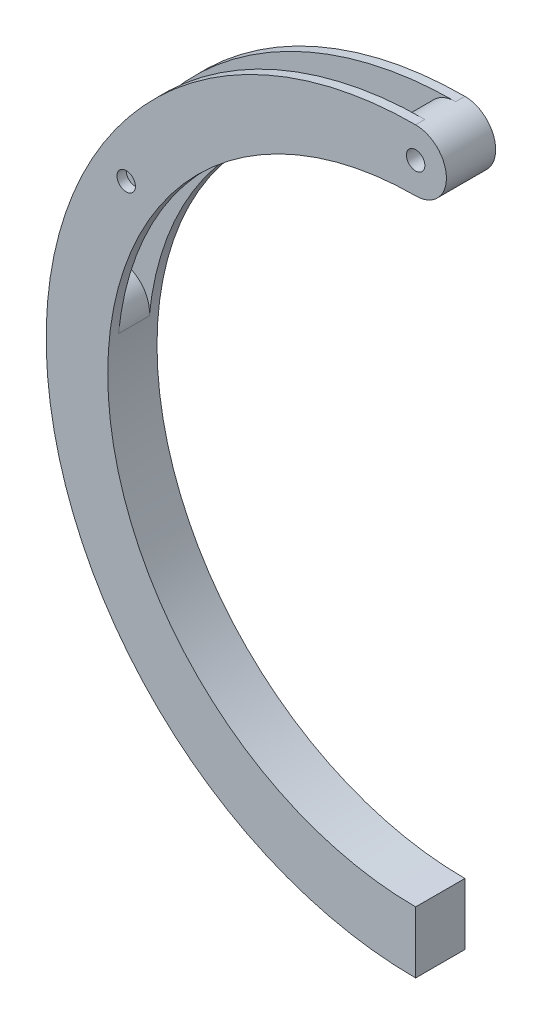
ISO-10303-21;
HEADER;
FILE_DESCRIPTION(('STEP AP214'),'2;1');
FILE_NAME('part.step','',(''),(''),'','','');
FILE_SCHEMA(('AUTOMOTIVE_DESIGN { 1 0 10303 214 1 1 1 1 }'));
ENDSEC;
DATA;
#1=APPLICATION_CONTEXT('core data for automotive mechanical design processes');
#2=APPLICATION_PROTOCOL_DEFINITION('international standard','automotive_design',2000,#1);
#3=PRODUCT_CONTEXT('',#1,'mechanical');
#4=PRODUCT('Part','Part','',(#3));
#5=PRODUCT_RELATED_PRODUCT_CATEGORY('part','',(#4));
#6=PRODUCT_DEFINITION_FORMATION('','',#4);
#7=PRODUCT_DEFINITION_CONTEXT('part definition',#1,'design');
#8=PRODUCT_DEFINITION('design','',#6,#7);
#9=PRODUCT_DEFINITION_SHAPE('','',#8);
#10=(LENGTH_UNIT() NAMED_UNIT(*) SI_UNIT(.MILLI.,.METRE.));
#11=(NAMED_UNIT(*) PLANE_ANGLE_UNIT() SI_UNIT($,.RADIAN.));
#12=(NAMED_UNIT(*) SI_UNIT($,.STERADIAN.) SOLID_ANGLE_UNIT());
#13=UNCERTAINTY_MEASURE_WITH_UNIT(LENGTH_MEASURE(1.E-05),#10,'distance_accuracy_value','');
#14=(GEOMETRIC_REPRESENTATION_CONTEXT(3) GLOBAL_UNCERTAINTY_ASSIGNED_CONTEXT((#13)) GLOBAL_UNIT_ASSIGNED_CONTEXT((#10,
#11,#12)) REPRESENTATION_CONTEXT('',''));
#15=CARTESIAN_POINT('',(0.,0.,0.));
#16=DIRECTION('',(0.,0.,1.));
#17=DIRECTION('',(1.,0.,0.));
#18=AXIS2_PLACEMENT_3D('',#15,#16,#17);
#19=CARTESIAN_POINT('',(0.,0.,4.));
#20=DIRECTION('',(0.,0.,1.));
#21=DIRECTION('',(1.,0.,0.));
#22=AXIS2_PLACEMENT_3D('',#19,#20,#21);
#23=PLANE('',#22);
#24=CARTESIAN_POINT('',(-47.,28.5657137141714,4.));
#25=DIRECTION('',(0.,0.,1.));
#26=DIRECTION('',(1.,0.,0.));
#27=AXIS2_PLACEMENT_3D('',#24,#25,#26);
#28=CIRCLE('',#27,1.5);
#29=CARTESIAN_POINT('',(-45.5,28.5657137141714,4.));
#30=VERTEX_POINT('',#29);
#31=EDGE_CURVE('E125',#30,#30,#28,.T.);
#32=ORIENTED_EDGE('',*,*,#31,.F.);
#33=EDGE_LOOP('',(#32));
#34=FACE_BOUND('',#33,.T.);
#35=CARTESIAN_POINT('',(0.,0.,4.));
#36=DIRECTION('',(0.,0.,1.));
#37=DIRECTION('',(1.,0.,0.));
#38=AXIS2_PLACEMENT_3D('',#35,#36,#37);
#39=CIRCLE('',#38,60.);
#40=CARTESIAN_POINT('',(0.,60.,4.));
#41=VERTEX_POINT('',#40);
#42=CARTESIAN_POINT('',(0.,-60.,4.));
#43=VERTEX_POINT('',#42);
#44=EDGE_CURVE('E123',#41,#43,#39,.T.);
#45=ORIENTED_EDGE('',*,*,#44,.T.);
#46=DIRECTION('',(0.,1.,0.));
#47=VECTOR('',#46,1.);
#48=CARTESIAN_POINT('',(0.,-50.,4.));
#49=LINE('',#48,#47);
#50=CARTESIAN_POINT('',(0.,-50.,4.));
#51=VERTEX_POINT('',#50);
#52=EDGE_CURVE('E186',#43,#51,#49,.T.);
#53=ORIENTED_EDGE('',*,*,#52,.T.);
#54=CARTESIAN_POINT('',(0.,0.,4.));
#55=DIRECTION('',(0.,0.,-1.));
#56=DIRECTION('',(1.,0.,0.));
#57=AXIS2_PLACEMENT_3D('',#54,#55,#56);
#58=CIRCLE('',#57,50.);
#59=CARTESIAN_POINT('',(0.,50.,4.));
#60=VERTEX_POINT('',#59);
#61=EDGE_CURVE('E150',#51,#60,#58,.T.);
#62=ORIENTED_EDGE('',*,*,#61,.T.);
#63=CARTESIAN_POINT('',(0.,55.,4.));
#64=DIRECTION('',(0.,0.,1.));
#65=DIRECTION('',(-1.,0.,0.));
#66=AXIS2_PLACEMENT_3D('',#63,#64,#65);
#67=CIRCLE('',#66,5.);
#68=EDGE_CURVE('E133',#60,#41,#67,.T.);
#69=ORIENTED_EDGE('',*,*,#68,.T.);
#70=EDGE_LOOP('',(#45,#53,#62,#69));
#71=FACE_BOUND('',#70,.T.);
#72=CARTESIAN_POINT('',(0.,55.,4.));
#73=DIRECTION('',(0.,0.,1.));
#74=DIRECTION('',(1.,0.,0.));
#75=AXIS2_PLACEMENT_3D('',#72,#73,#74);
#76=CIRCLE('',#75,1.5);
#77=CARTESIAN_POINT('',(1.5,55.,4.));
#78=VERTEX_POINT('',#77);
#79=EDGE_CURVE('E176',#78,#78,#76,.T.);
#80=ORIENTED_EDGE('',*,*,#79,.F.);
#81=EDGE_LOOP('',(#80));
#82=FACE_BOUND('',#81,.T.);
#83=ADVANCED_FACE('F39',(#34,#71,#82),#23,.T.);
#84=CARTESIAN_POINT('',(0.,0.,2.5));
#85=DIRECTION('',(0.,0.,1.));
#86=DIRECTION('',(1.,0.,0.));
#87=AXIS2_PLACEMENT_3D('',#84,#85,#86);
#88=PLANE('',#87);
#89=CARTESIAN_POINT('',(-54.7247707207909,5.49540440339574,2.5));
#90=DIRECTION('',(0.,0.,1.));
#91=DIRECTION('',(1.,0.,0.));
#92=AXIS2_PLACEMENT_3D('',#89,#90,#91);
#93=CIRCLE('',#92,4.99999999999999);
#94=CARTESIAN_POINT('',(-49.7497915643554,4.99582218490522,2.5));
#95=VERTEX_POINT('',#94);
#96=CARTESIAN_POINT('',(-59.6997498772265,5.99498662188626,2.5));
#97=VERTEX_POINT('',#96);
#98=EDGE_CURVE('E53',#95,#97,#93,.T.);
#99=ORIENTED_EDGE('',*,*,#98,.T.);
#100=CARTESIAN_POINT('',(0.,0.,2.5));
#101=DIRECTION('',(0.,0.,1.));
#102=DIRECTION('',(1.,0.,0.));
#103=AXIS2_PLACEMENT_3D('',#100,#101,#102);
#104=CIRCLE('',#103,60.);
#105=CARTESIAN_POINT('',(0.,60.,2.5));
#106=VERTEX_POINT('',#105);
#107=EDGE_CURVE('E113',#106,#97,#104,.T.);
#108=ORIENTED_EDGE('',*,*,#107,.F.);
#109=CARTESIAN_POINT('',(0.,55.,2.5));
#110=DIRECTION('',(0.,0.,1.));
#111=DIRECTION('',(1.,0.,0.));
#112=AXIS2_PLACEMENT_3D('',#109,#110,#111);
#113=CIRCLE('',#112,5.);
#114=CARTESIAN_POINT('',(0.,50.,2.5));
#115=VERTEX_POINT('',#114);
#116=EDGE_CURVE('E179',#106,#115,#113,.T.);
#117=ORIENTED_EDGE('',*,*,#116,.T.);
#118=CARTESIAN_POINT('',(0.,0.,2.5));
#119=DIRECTION('',(0.,0.,-1.));
#120=DIRECTION('',(1.,0.,0.));
#121=AXIS2_PLACEMENT_3D('',#118,#119,#120);
#122=CIRCLE('',#121,50.);
#123=EDGE_CURVE('E118',#95,#115,#122,.T.);
#124=ORIENTED_EDGE('',*,*,#123,.F.);
#125=EDGE_LOOP('',(#99,#108,#117,#124));
#126=FACE_BOUND('',#125,.T.);
#127=CARTESIAN_POINT('',(-47.,28.5657137141714,2.5));
#128=DIRECTION('',(0.,0.,1.));
#129=DIRECTION('',(1.,0.,0.));
#130=AXIS2_PLACEMENT_3D('',#127,#128,#129);
#131=CIRCLE('',#130,1.5);
#132=CARTESIAN_POINT('',(-45.5,28.5657137141714,2.5));
#133=VERTEX_POINT('',#132);
#134=EDGE_CURVE('E126',#133,#133,#131,.T.);
#135=ORIENTED_EDGE('',*,*,#134,.T.);
#136=EDGE_LOOP('',(#135));
#137=FACE_BOUND('',#136,.T.);
#138=ADVANCED_FACE('F115',(#126,#137),#88,.F.);
#139=CARTESIAN_POINT('',(0.,0.,4.));
#140=DIRECTION('',(0.,0.,-1.));
#141=DIRECTION('',(-1.,0.,0.));
#142=AXIS2_PLACEMENT_3D('',#139,#140,#141);
#143=CYLINDRICAL_SURFACE('',#142,60.);
#144=ORIENTED_EDGE('',*,*,#107,.T.);
#145=DIRECTION('',(0.,0.,-1.));
#146=VECTOR('',#145,1.);
#147=CARTESIAN_POINT('',(-59.6997498772265,5.99498662188626,95.0721450653398));
#148=LINE('',#147,#146);
#149=CARTESIAN_POINT('',(-59.6997498772265,5.99498662188626,-2.5));
#150=VERTEX_POINT('',#149);
#151=EDGE_CURVE('E105',#97,#150,#148,.T.);
#152=ORIENTED_EDGE('',*,*,#151,.T.);
#153=CARTESIAN_POINT('',(0.,0.,-2.5));
#154=DIRECTION('',(0.,0.,1.));
#155=DIRECTION('',(1.,0.,0.));
#156=AXIS2_PLACEMENT_3D('',#153,#154,#155);
#157=CIRCLE('',#156,60.);
#158=CARTESIAN_POINT('',(0.,60.,-2.5));
#159=VERTEX_POINT('',#158);
#160=EDGE_CURVE('E65',#159,#150,#157,.T.);
#161=ORIENTED_EDGE('',*,*,#160,.F.);
#162=DIRECTION('',(0.,0.,1.));
#163=VECTOR('',#162,1.);
#164=CARTESIAN_POINT('',(0.,60.,-4.));
#165=LINE('',#164,#163);
#166=CARTESIAN_POINT('',(0.,60.,-4.));
#167=VERTEX_POINT('',#166);
#168=EDGE_CURVE('E175',#167,#159,#165,.T.);
#169=ORIENTED_EDGE('',*,*,#168,.F.);
#170=CARTESIAN_POINT('',(0.,0.,-4.));
#171=DIRECTION('',(0.,0.,1.));
#172=DIRECTION('',(1.,0.,0.));
#173=AXIS2_PLACEMENT_3D('',#170,#171,#172);
#174=CIRCLE('',#173,60.);
#175=CARTESIAN_POINT('',(0.,-60.,-4.));
#176=VERTEX_POINT('',#175);
#177=EDGE_CURVE('E161',#167,#176,#174,.T.);
#178=ORIENTED_EDGE('',*,*,#177,.T.);
#179=DIRECTION('',(0.,0.,-1.));
#180=VECTOR('',#179,1.);
#181=CARTESIAN_POINT('',(0.,-60.,4.));
#182=LINE('',#181,#180);
#183=EDGE_CURVE('E11',#43,#176,#182,.T.);
#184=ORIENTED_EDGE('',*,*,#183,.F.);
#185=ORIENTED_EDGE('',*,*,#44,.F.);
#186=DIRECTION('',(0.,0.,-1.));
#187=VECTOR('',#186,1.);
#188=CARTESIAN_POINT('',(0.,60.,4.));
#189=LINE('',#188,#187);
#190=EDGE_CURVE('E124',#41,#106,#189,.T.);
#191=ORIENTED_EDGE('',*,*,#190,.T.);
#192=EDGE_LOOP('',(#144,#152,#161,#169,#178,#184,#185,#191));
#193=FACE_BOUND('',#192,.T.);
#194=ADVANCED_FACE('F41',(#193),#143,.T.);
#195=CARTESIAN_POINT('',(0.,-50.,4.));
#196=DIRECTION('',(-1.,0.,0.));
#197=DIRECTION('',(0.,0.,1.));
#198=AXIS2_PLACEMENT_3D('',#195,#196,#197);
#199=PLANE('',#198);
#200=ORIENTED_EDGE('',*,*,#183,.T.);
#201=DIRECTION('',(0.,1.,0.));
#202=VECTOR('',#201,1.);
#203=CARTESIAN_POINT('',(0.,-50.,-4.));
#204=LINE('',#203,#202);
#205=CARTESIAN_POINT('',(0.,-50.,-4.));
#206=VERTEX_POINT('',#205);
#207=EDGE_CURVE('E152',#176,#206,#204,.T.);
#208=ORIENTED_EDGE('',*,*,#207,.T.);
#209=DIRECTION('',(0.,0.,-1.));
#210=VECTOR('',#209,1.);
#211=CARTESIAN_POINT('',(0.,-50.,4.));
#212=LINE('',#211,#210);
#213=EDGE_CURVE('E50',#51,#206,#212,.T.);
#214=ORIENTED_EDGE('',*,*,#213,.F.);
#215=ORIENTED_EDGE('',*,*,#52,.F.);
#216=EDGE_LOOP('',(#200,#208,#214,#215));
#217=FACE_BOUND('',#216,.T.);
#218=ADVANCED_FACE('F157',(#217),#199,.F.);
#219=CARTESIAN_POINT('',(0.,0.,4.));
#220=DIRECTION('',(0.,0.,-1.));
#221=DIRECTION('',(-1.,0.,0.));
#222=AXIS2_PLACEMENT_3D('',#219,#220,#221);
#223=CYLINDRICAL_SURFACE('',#222,50.);
#224=ORIENTED_EDGE('',*,*,#213,.T.);
#225=CARTESIAN_POINT('',(0.,0.,-4.));
#226=DIRECTION('',(0.,0.,-1.));
#227=DIRECTION('',(1.,0.,0.));
#228=AXIS2_PLACEMENT_3D('',#225,#226,#227);
#229=CIRCLE('',#228,50.);
#230=CARTESIAN_POINT('',(0.,50.,-4.));
#231=VERTEX_POINT('',#230);
#232=EDGE_CURVE('E145',#206,#231,#229,.T.);
#233=ORIENTED_EDGE('',*,*,#232,.T.);
#234=DIRECTION('',(0.,0.,1.));
#235=VECTOR('',#234,1.);
#236=CARTESIAN_POINT('',(0.,50.,-4.));
#237=LINE('',#236,#235);
#238=CARTESIAN_POINT('',(0.,50.,-2.5));
#239=VERTEX_POINT('',#238);
#240=EDGE_CURVE('E169',#231,#239,#237,.T.);
#241=ORIENTED_EDGE('',*,*,#240,.T.);
#242=CARTESIAN_POINT('',(0.,0.,-2.5));
#243=DIRECTION('',(0.,0.,-1.));
#244=DIRECTION('',(1.,0.,0.));
#245=AXIS2_PLACEMENT_3D('',#242,#243,#244);
#246=CIRCLE('',#245,50.);
#247=CARTESIAN_POINT('',(-49.7497915643554,4.99582218490522,-2.5));
#248=VERTEX_POINT('',#247);
#249=EDGE_CURVE('E162',#248,#239,#246,.T.);
#250=ORIENTED_EDGE('',*,*,#249,.F.);
#251=DIRECTION('',(0.,0.,-1.));
#252=VECTOR('',#251,1.);
#253=CARTESIAN_POINT('',(-49.7497915643554,4.99582218490522,95.0721450653398));
#254=LINE('',#253,#252);
#255=EDGE_CURVE('E110',#95,#248,#254,.T.);
#256=ORIENTED_EDGE('',*,*,#255,.F.);
#257=ORIENTED_EDGE('',*,*,#123,.T.);
#258=DIRECTION('',(0.,0.,-1.));
#259=VECTOR('',#258,1.);
#260=CARTESIAN_POINT('',(0.,50.,4.));
#261=LINE('',#260,#259);
#262=EDGE_CURVE('E132',#60,#115,#261,.T.);
#263=ORIENTED_EDGE('',*,*,#262,.F.);
#264=ORIENTED_EDGE('',*,*,#61,.F.);
#265=EDGE_LOOP('',(#224,#233,#241,#250,#256,#257,#263,#264));
#266=FACE_BOUND('',#265,.T.);
#267=ADVANCED_FACE('F142',(#266),#223,.F.);
#268=CARTESIAN_POINT('',(0.,55.,4.));
#269=DIRECTION('',(0.,0.,-1.));
#270=DIRECTION('',(-1.,0.,0.));
#271=AXIS2_PLACEMENT_3D('',#268,#269,#270);
#272=CYLINDRICAL_SURFACE('',#271,5.);
#273=ORIENTED_EDGE('',*,*,#262,.T.);
#274=ORIENTED_EDGE('',*,*,#116,.F.);
#275=ORIENTED_EDGE('',*,*,#190,.F.);
#276=ORIENTED_EDGE('',*,*,#68,.F.);
#277=EDGE_LOOP('',(#273,#274,#275,#276));
#278=FACE_BOUND('',#277,.T.);
#279=CARTESIAN_POINT('',(0.,55.,-2.5));
#280=DIRECTION('',(0.,0.,1.));
#281=DIRECTION('',(1.,0.,0.));
#282=AXIS2_PLACEMENT_3D('',#279,#280,#281);
#283=CIRCLE('',#282,5.);
#284=EDGE_CURVE('E172',#159,#239,#283,.T.);
#285=ORIENTED_EDGE('',*,*,#284,.T.);
#286=ORIENTED_EDGE('',*,*,#240,.F.);
#287=CARTESIAN_POINT('',(0.,55.,-4.));
#288=DIRECTION('',(0.,0.,1.));
#289=DIRECTION('',(-1.,0.,0.));
#290=AXIS2_PLACEMENT_3D('',#287,#288,#289);
#291=CIRCLE('',#290,5.);
#292=EDGE_CURVE('E160',#231,#167,#291,.T.);
#293=ORIENTED_EDGE('',*,*,#292,.T.);
#294=ORIENTED_EDGE('',*,*,#168,.T.);
#295=EDGE_LOOP('',(#285,#286,#293,#294));
#296=FACE_BOUND('',#295,.T.);
#297=ADVANCED_FACE('F195',(#278,#296),#272,.T.);
#298=CARTESIAN_POINT('',(-47.,28.5657137141714,4.));
#299=DIRECTION('',(0.,0.,-1.));
#300=DIRECTION('',(-1.,0.,0.));
#301=AXIS2_PLACEMENT_3D('',#298,#299,#300);
#302=CYLINDRICAL_SURFACE('',#301,1.5);
#303=ORIENTED_EDGE('',*,*,#31,.T.);
#304=EDGE_LOOP('',(#303));
#305=FACE_BOUND('',#304,.T.);
#306=ORIENTED_EDGE('',*,*,#134,.F.);
#307=EDGE_LOOP('',(#306));
#308=FACE_BOUND('',#307,.T.);
#309=ADVANCED_FACE('F217',(#305,#308),#302,.F.);
#310=CARTESIAN_POINT('',(0.,55.,4.));
#311=DIRECTION('',(0.,0.,-1.));
#312=DIRECTION('',(-1.,0.,0.));
#313=AXIS2_PLACEMENT_3D('',#310,#311,#312);
#314=CYLINDRICAL_SURFACE('',#313,1.5);
#315=ORIENTED_EDGE('',*,*,#79,.T.);
#316=EDGE_LOOP('',(#315));
#317=FACE_BOUND('',#316,.T.);
#318=CARTESIAN_POINT('',(0.,55.,-4.));
#319=DIRECTION('',(0.,0.,1.));
#320=DIRECTION('',(1.,0.,0.));
#321=AXIS2_PLACEMENT_3D('',#318,#319,#320);
#322=CIRCLE('',#321,1.5);
#323=CARTESIAN_POINT('',(1.5,55.,-4.));
#324=VERTEX_POINT('',#323);
#325=EDGE_CURVE('E120',#324,#324,#322,.T.);
#326=ORIENTED_EDGE('',*,*,#325,.F.);
#327=EDGE_LOOP('',(#326));
#328=FACE_BOUND('',#327,.T.);
#329=ADVANCED_FACE('F209',(#317,#328),#314,.F.);
#330=CARTESIAN_POINT('',(0.,0.,-2.5));
#331=DIRECTION('',(0.,0.,1.));
#332=DIRECTION('',(1.,0.,0.));
#333=AXIS2_PLACEMENT_3D('',#330,#331,#332);
#334=PLANE('',#333);
#335=CARTESIAN_POINT('',(-47.,28.5657137141714,-2.5));
#336=DIRECTION('',(0.,0.,1.));
#337=DIRECTION('',(1.,0.,0.));
#338=AXIS2_PLACEMENT_3D('',#335,#336,#337);
#339=CIRCLE('',#338,1.5);
#340=CARTESIAN_POINT('',(-45.5,28.5657137141714,-2.5));
#341=VERTEX_POINT('',#340);
#342=EDGE_CURVE('E203',#341,#341,#339,.T.);
#343=ORIENTED_EDGE('',*,*,#342,.F.);
#344=EDGE_LOOP('',(#343));
#345=FACE_BOUND('',#344,.T.);
#346=ORIENTED_EDGE('',*,*,#160,.T.);
#347=CARTESIAN_POINT('',(-54.7247707207909,5.49540440339574,-2.5));
#348=DIRECTION('',(0.,0.,1.));
#349=DIRECTION('',(-1.,0.,0.));
#350=AXIS2_PLACEMENT_3D('',#347,#348,#349);
#351=CIRCLE('',#350,4.99999999999999);
#352=EDGE_CURVE('E102',#248,#150,#351,.T.);
#353=ORIENTED_EDGE('',*,*,#352,.F.);
#354=ORIENTED_EDGE('',*,*,#249,.T.);
#355=ORIENTED_EDGE('',*,*,#284,.F.);
#356=EDGE_LOOP('',(#346,#353,#354,#355));
#357=FACE_BOUND('',#356,.T.);
#358=ADVANCED_FACE('F208',(#345,#357),#334,.T.);
#359=CARTESIAN_POINT('',(0.,0.,-4.));
#360=DIRECTION('',(0.,0.,1.));
#361=DIRECTION('',(1.,0.,0.));
#362=AXIS2_PLACEMENT_3D('',#359,#360,#361);
#363=PLANE('',#362);
#364=ORIENTED_EDGE('',*,*,#325,.T.);
#365=EDGE_LOOP('',(#364));
#366=FACE_BOUND('',#365,.T.);
#367=CARTESIAN_POINT('',(-47.,28.5657137141714,-4.));
#368=DIRECTION('',(0.,0.,1.));
#369=DIRECTION('',(1.,0.,0.));
#370=AXIS2_PLACEMENT_3D('',#367,#368,#369);
#371=CIRCLE('',#370,1.5);
#372=CARTESIAN_POINT('',(-45.5,28.5657137141714,-4.));
#373=VERTEX_POINT('',#372);
#374=EDGE_CURVE('E168',#373,#373,#371,.T.);
#375=ORIENTED_EDGE('',*,*,#374,.T.);
#376=EDGE_LOOP('',(#375));
#377=FACE_BOUND('',#376,.T.);
#378=ORIENTED_EDGE('',*,*,#177,.F.);
#379=ORIENTED_EDGE('',*,*,#292,.F.);
#380=ORIENTED_EDGE('',*,*,#232,.F.);
#381=ORIENTED_EDGE('',*,*,#207,.F.);
#382=EDGE_LOOP('',(#378,#379,#380,#381));
#383=FACE_BOUND('',#382,.T.);
#384=ADVANCED_FACE('F153',(#366,#377,#383),#363,.F.);
#385=CARTESIAN_POINT('',(-47.,28.5657137141714,-4.));
#386=DIRECTION('',(0.,0.,1.));
#387=DIRECTION('',(1.,0.,0.));
#388=AXIS2_PLACEMENT_3D('',#385,#386,#387);
#389=CYLINDRICAL_SURFACE('',#388,1.5);
#390=ORIENTED_EDGE('',*,*,#374,.F.);
#391=EDGE_LOOP('',(#390));
#392=FACE_BOUND('',#391,.T.);
#393=ORIENTED_EDGE('',*,*,#342,.T.);
#394=EDGE_LOOP('',(#393));
#395=FACE_BOUND('',#394,.T.);
#396=ADVANCED_FACE('F206',(#392,#395),#389,.F.);
#397=CARTESIAN_POINT('',(-54.7247707207909,5.49540440339574,95.0721450653398));
#398=DIRECTION('',(0.,0.,-1.));
#399=DIRECTION('',(-1.,0.,0.));
#400=AXIS2_PLACEMENT_3D('',#397,#398,#399);
#401=CYLINDRICAL_SURFACE('',#400,4.99999999999999);
#402=ORIENTED_EDGE('',*,*,#98,.F.);
#403=ORIENTED_EDGE('',*,*,#255,.T.);
#404=ORIENTED_EDGE('',*,*,#352,.T.);
#405=ORIENTED_EDGE('',*,*,#151,.F.);
#406=EDGE_LOOP('',(#402,#403,#404,#405));
#407=FACE_BOUND('',#406,.T.);
#408=ADVANCED_FACE('F103',(#407),#401,.T.);
#409=CLOSED_SHELL('',(#83,#138,#194,#218,#267,#297,#309,#329,#358,#384,#396,#408));
#410=MANIFOLD_SOLID_BREP('B2',#409);
#411=ADVANCED_BREP_SHAPE_REPRESENTATION('',(#18,#410),#14);
#412=SHAPE_DEFINITION_REPRESENTATION(#9,#411);
ENDSEC;
END-ISO-10303-21;
